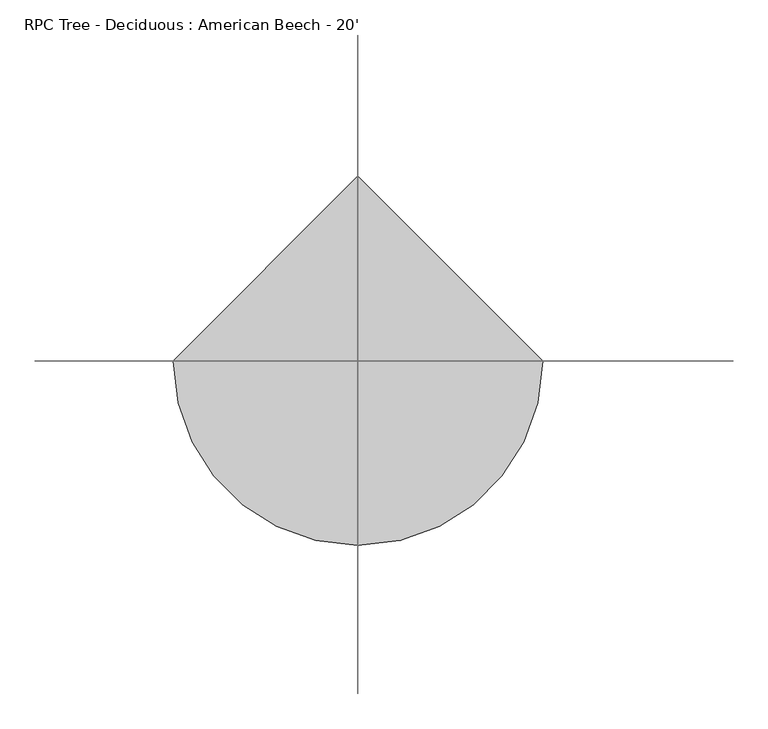
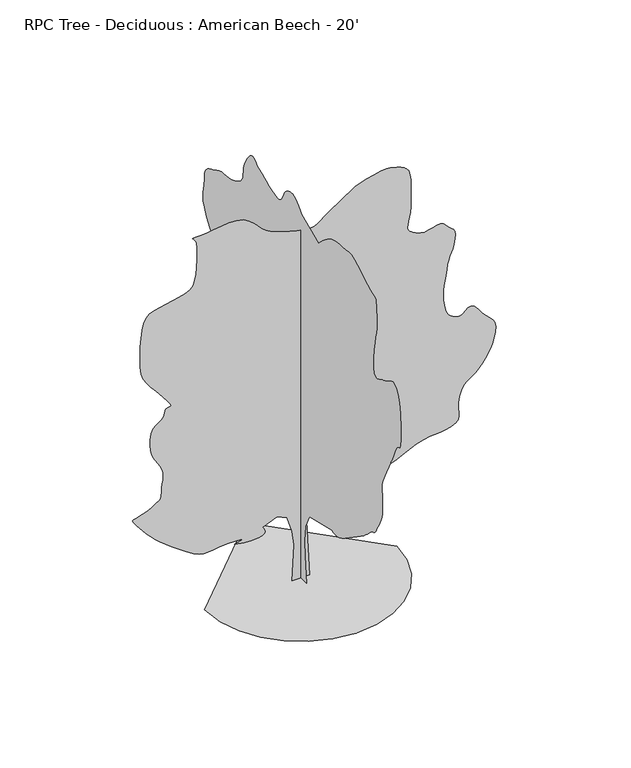
"""IFC4 building model written with IfcOpenShell, lengths in millimetres: geographic element geometry, RPC Tree - Deciduous : American Beech - 20'."""

from ifc_helpers import new_model, si_unit, origin, place, context, project, spatial, triangles, source, transform, mapped, element, save


def rpc_tree_deciduous_american_beech_20_b3c041c8(model_context):
    return source(origin(), model_context, "Body", "Tessellation", [
        triangles([(0.0009889, 136.856581, 0.0), (0.0009889, -149.8547884, 0.0), (0.0009889, -111.6264895, 420.510052), (0.0009889, -102.0697236, 659.4353302), (0.0009889, -121.1832463, 898.3606447), (0.0009889, -235.8678885, 1118.172373), (0.0009889, -818.8458761, 1261.5275036), (0.0009889, -849.9431059, 1249.7139805), (0.0009889, -883.2933231, 1240.7427258), (0.0009889, -921.1596891, 1237.4533916), (0.0009889, -965.7976622, 1242.6934788), (0.0009889, -1019.4603024, 1259.3000233), (0.0009889, -1084.4081549, 1290.1152935), (0.0009889, -1162.8992941, 1337.984174), (0.0009889, -1478.2811337, 1557.7959023), (0.0009889, -1522.8632961, 1589.1420994), (0.0009889, -1566.942437, 1618.9819931), (0.0009889, -1611.1893002, 1649.3249084), (0.0009889, -1656.2718681, 1682.1772636), (0.0009889, -1702.8579781, 1719.5406807), (0.0009889, -1751.6183739, 1763.4243393), (0.0009889, -1803.2210381, 1815.834803), (0.0009889, -1847.9404015, 1858.0191467), (0.0009889, -1878.9512993, 1877.1351311), (0.0009889, -1901.2702858, 1884.0440117), (0.0009889, -1919.9112991, 1889.616782), (0.0009889, -1939.8884228, 1904.7196392), (0.0009889, -1966.2180656, 1940.2161644), (0.0009889, -2003.916782, 2006.9774963), (0.0009889, -2044.9607883, 2083.2080177), (0.0009889, -2078.313549, 2145.2324295), (0.0009889, -2104.4754696, 2201.0692829), (0.0009889, -2123.9521877, 2258.7475937), (0.0009889, -2137.244109, 2326.2862038), (0.0009889, -2144.8488773, 2411.7141289), (0.0009889, -2147.2746014, 2523.0550072), (0.0009889, -2142.5373905, 2624.8889076), (0.0009889, -2132.7863869, 2688.2873634), (0.0009889, -2124.7040314, 2730.9338882), (0.0009889, -2124.9835201, 2770.583503), (0.0009889, -2140.3072941, 2824.9394875), (0.0009889, -2177.3659332, 2911.7568626), (0.0009889, -2242.84464, 3048.6883301), (0.0009889, -2308.7119858, 3181.9621719), (0.0009889, -2348.5011269, 3259.3812836), (0.0009889, -2371.2366577, 3301.215358), (0.0009889, -2385.9484051, 3327.6567673), (0.0009889, -2401.6632889, 3358.9496246), (0.0009889, -2427.4088104, 3415.3121727), (0.0009889, -2472.2118896, 3516.9885246), (0.0009889, -2522.8114174, 3609.6476944), (0.0009889, -2561.0332123, 3645.1568642), (0.0009889, -2588.5669968, 3652.9040657), (0.0009889, -2607.0580193, 3662.3273277), (0.0009889, -2618.2087921, 3702.8402618), (0.0009889, -2623.669796, 3803.856189), (0.0009889, -2625.117382, 3994.8390083), (0.0009889, -2615.3639076, 4210.713913), (0.0009889, -2589.2271309, 4371.4450905), (0.0009889, -2551.406765, 4483.8402649), (0.0009889, -2506.5400269, 4554.7824463), (0.0009889, -2459.3391289, 4591.1043571), (0.0009889, -2414.4802391, 4599.6895889), (0.0009889, -2376.641851, 4587.3705734), (0.0009889, -2343.8477772, 4566.9491455), (0.0009889, -2310.8862717, 4546.8576393), (0.0009889, -2277.5893215, 4527.4521378), (0.0009889, -2243.7921112, 4509.0116936), (0.0009889, -2209.3243023, 4491.9426773), (0.0009889, -2174.0232594, 4476.5250137), (0.0009889, -2137.7164639, 4463.1392029), (0.0009889, -2096.4236355, 4443.6572525), (0.0009889, -2049.6139927, 4418.4858238), (0.0009889, -2002.3013283, 4400.6805153), (0.0009889, -1959.504958, 4403.2713455), (0.0009889, -1926.2359131, 4439.313913), (0.0009889, -1907.5110386, 4521.8132378), (0.0009889, -1908.3467434, 4663.8246277), (0.0009889, -1923.6450829, 4819.4253044), (0.0009889, -1942.954224, 4940.7356323), (0.0009889, -1963.266647, 5037.9669067), (0.0009889, -1981.572361, 5121.3298416), (0.0009889, -1994.8642822, 5201.0354416), (0.0009889, -2000.1296585, 5287.2429703), (0.0009889, -1994.3614059, 5390.1634323), (0.0009889, -1986.3653824, 5488.9190323), (0.0009889, -1983.048143, 5559.911792), (0.0009889, -1978.5625156, 5609.3407516), (0.0009889, -1967.0562412, 5643.3764648), (0.0009889, -1942.6748806, 5668.2429703), (0.0009889, -1899.5709709, 5690.0869858), (0.0009889, -1831.8926891, 5715.1063889), (0.0009889, -1748.4408062, 5751.9616974), (0.0009889, -1662.820015, 5800.5261749), (0.0009889, -1576.3582867, 5853.7903656), (0.0009889, -1490.4020508, 5904.6919098), (0.0009889, -1406.2848015, 5946.2207703), (0.0009889, -1325.3426491, 5971.3924896), (0.0009889, -1248.913884, 5973.1447083), (0.0009889, -1174.2403896, 5963.3406555), (0.0009889, -1098.5636135, 5956.711409), (0.0009889, -1023.222064, 5950.5641098), (0.0009889, -949.5518515, 5942.2588028), (0.0009889, -878.8914843, 5929.1264648), (0.0009889, -812.5771454, 5908.4509827), (0.0009889, -751.9472706, 5877.5644958), (0.0009889, -697.9494038, 5841.2678741), (0.0009889, -649.9687569, 5805.9618896), (0.0009889, -607.0045916, 5771.4942261), (0.0009889, -568.0511189, 5737.7119858), (0.0009889, -532.1075644, 5704.4128555), (0.0009889, -498.1706097, 5671.4433563), (0.0009889, -465.2369368, 5638.6523346), (0.0009889, -16.056217, 5829.7871796), (0.0009889, 22.8405617, 5872.4339951), (0.0009889, 61.6537222, 5913.023378), (0.0009889, 100.2998553, 5949.3961578), (0.0009889, 138.6950317, 5979.5204819), (0.0009889, 176.7559443, 6001.2883392), (0.0009889, 214.3990318, 6012.5911377), (0.0009889, 251.5404602, 6011.3720261), (0.0009889, 287.2056524, 6002.4312927), (0.0009889, 320.3628219, 5991.305809), (0.0009889, 350.8454089, 5977.0055191), (0.0009889, 378.4856913, 5958.5397858), (0.0009889, 403.1160919, 5934.892392), (0.0009889, 424.5689612, 5905.047702), (0.0009889, 442.6817001, 5868.0144974), (0.0009889, 459.9562634, 5826.9425858), (0.0009889, 480.2407084, 5787.547316), (0.0009889, 505.3740581, 5752.6727005), (0.0009889, 537.1926464, 5725.138916), (0.0009889, 577.5380399, 5707.7911377), (0.0009889, 628.2491524, 5703.5239563), (0.0009889, 691.1650068, 5715.1063889), (0.0009889, 759.6790661, 5736.9754028), (0.0009889, 826.1890326, 5761.3593796), (0.0009889, 891.0251186, 5787.8263687), (0.0009889, 954.5251671, 5815.9694183), (0.0009889, 1017.0218611, 5845.3577408), (0.0009889, 1078.8506453, 5875.5832214), (0.0009889, 1140.3440575, 5906.2412338), (0.0009889, 1169.0715191, 5932.3524307), (0.0009889, 1198.1316639, 5955.3649796), (0.0009889, 1227.8624073, 5972.2052307), (0.0009889, 1258.5938164, 5979.7489563), (0.0009889, 1290.6664227, 5974.9230881), (0.0009889, 1324.4078224, 5954.6539764), (0.0009889, 1360.1557858, 5915.7918137), (0.0009889, 1395.1799561, 5868.217392), (0.0009889, 1426.1908539, 5822.9544571), (0.0009889, 1452.6880737, 5778.8856354), (0.0009889, 1474.1715008, 5734.7912338), (0.0009889, 1490.1379681, 5689.5538788), (0.0009889, 1500.0845993, 5641.9538773), (0.0009889, 1503.510989, 5590.8494385), (0.0009889, 1507.2168674, 5539.3380478), (0.0009889, 1519.1142517, 5491.1793594), (0.0009889, 1540.3740005, 5446.1704788), (0.0009889, 1572.1672634, 5404.1846695), (0.0009889, 1615.6596668, 5365.0428726), (0.0009889, 1672.0274471, 5328.5689362), (0.0009889, 1742.4363762, 5294.5832199), (0.0009889, 1817.5288857, 5269.1836075), (0.0009889, 1887.9378147, 5255.1373718), (0.0009889, 1954.8363476, 5247.4407486), (0.0009889, 2019.3956337, 5241.0911362), (0.0009889, 2082.7839157, 5231.0580276), (0.0009889, 2146.1721977, 5212.3382401), (0.0009889, 2210.7313385, 5179.9024292), (0.0009889, 2276.3498623, 5145.3580261), (0.0009889, 2340.1267834, 5118.8404587), (0.0009889, 2399.0573433, 5093.1356323), (0.0009889, 2450.1315514, 5061.106192), (0.0009889, 2490.3372368, 5015.5136261), (0.0009889, 2516.667025, 4949.193837), (0.0009889, 2526.1132507, 4854.9597633), (0.0009889, 2532.46577, 4758.008123), (0.0009889, 2546.5044479, 4681.9348595), (0.0009889, 2560.7285797, 4617.2411339), (0.0009889, 2567.5865913, 4554.3760757), (0.0009889, 2559.5600464, 4483.8402649), (0.0009889, 2529.1232414, 4396.0578323), (0.0009889, 2468.7702393, 4281.5543564), (0.0009889, 2394.0992157, 4166.6192207), (0.0009889, 2326.6139454, 4078.2525215), (0.0009889, 2267.6553349, 4007.9707649), (0.0009889, 2218.5596397, 3947.1884285), (0.0009889, 2180.6679119, 3887.4223091), (0.0009889, 2155.3111748, 3820.1377533), (0.0009889, 2143.8328056, 3736.8001076), (0.0009889, 2149.4334812, 3646.0204742), (0.0009889, 2171.0820145, 3561.7686401), (0.0009889, 2203.7667927, 3483.5112076), (0.0009889, 2242.4687908, 3410.790937), (0.0009889, 2282.1714546, 3343.1000107), (0.0009889, 2317.8662235, 3279.9047401), (0.0009889, 2344.5311657, 3220.7225967), (0.0009889, 2370.3577869, 3180.6921913), (0.0009889, 2402.5396889, 3164.8934464), (0.0009889, 2434.5538685, 3157.7813805), (0.0009889, 2459.8827003, 3143.8113029), (0.0009889, 2472.0037628, 3107.4638123), (0.0009889, 2464.3963783, 3033.1433487), (0.0009889, 2430.5432121, 2905.3305107), (0.0009889, 2383.9011463, 2761.3378464), (0.0009889, 2340.6017544, 2643.9136185), (0.0009889, 2298.1379219, 2545.7425758), (0.0009889, 2254.0028252, 2459.415287), (0.0009889, 2205.6894951, 2377.6095245), (0.0009889, 2150.6857304, 2292.9614937), (0.0009889, 2086.4897942, 2198.1177189), (0.0009889, 2022.098085, 2102.5196297), (0.0009889, 1968.0723129, 2019.6267242), (0.0009889, 1924.2446102, 1948.102747), (0.0009889, 1890.4447838, 1886.6067913), (0.0009889, 1866.5103436, 1833.8078339), (0.0009889, 1852.2735672, 1788.3620613), (0.0009889, 1847.564407, 1748.9361248), (0.0009889, 1851.5776794, 1721.8800728), (0.0009889, 1860.940044, 1709.2029396), (0.0009889, 1871.6386642, 1703.0459026), (0.0009889, 1879.6624477, 1695.5504299), (0.0009889, 1881.0010288, 1678.8600243), (0.0009889, 1871.6386642, 1645.1186245), (0.0009889, 1847.564407, 1586.4675533), (0.0009889, 1827.5314728, 1524.5828133), (0.0009889, 1825.3850922, 1482.2587978), (0.0009889, 1829.7590984, 1453.3104195), (0.0009889, 1829.2865982, 1431.547649), (0.0009889, 1812.5961926, 1410.7907764), (0.0009889, 1768.3214241, 1384.8497726), (0.0009889, 1685.0958355, 1347.5421661), (0.0009889, 1594.399918, 1309.4244347), (0.0009889, 1528.281134, 1282.5080544), (0.0009889, 1476.2059696, 1262.7823689), (0.0009889, 1427.6412014, 1246.2316349), (0.0009889, 1372.05317, 1228.8453415), (0.0009889, 1298.9138844, 1206.6102161), (0.0009889, 1197.6871416, 1175.5154572), (0.0009889, 1096.069289, 1145.7009253), (0.0009889, 1022.5387482, 1127.7557997), (0.0009889, 967.7331545, 1118.3400227), (0.0009889, 922.2874546, 1114.10329), (0.0009889, 876.8442255, 1111.7080873), (0.0009889, 822.0360884, 1107.806654), (0.0009889, 748.5055475, 1099.0588594), (0.0009889, 662.4935011, 1085.0990284), (0.0009889, 576.4788749, 1068.1292793), (0.0009889, 490.4667558, 1048.6551046), (0.0009889, 404.4521296, 1027.1717503), (0.0009889, 318.4400468, 1004.1847086), (0.0009889, 232.4266923, 980.1943851), (0.0009889, 146.4133378, 955.7037289), (136.1842383, 0.0003154, 0.014068), (-131.4120823, 0.0003154, 0.014068), (-102.7410489, 0.0002819, 563.8778998), (-131.4120823, 0.0002692, 793.2477293), (-207.8684348, 0.0002549, 1032.1729712), (-360.7819027, 0.0002501, 1108.6296415), (-580.5936673, 0.0002549, 1013.0594576), (-562.704425, 0.0002564, 988.5662579), (-548.0765751, 0.000258, 964.5784779), (-539.9688578, 0.0002596, 941.5914362), (-541.6401947, 0.0002612, 920.1080818), (-556.3518694, 0.0002628, 900.6313637), (-587.3627672, 0.0002628, 883.6641581), (-637.9342443, 0.0002644, 869.704327), (-697.421093, 0.0002644, 860.4815615), (-753.4001616, 0.0002644, 856.775683), (-806.4506298, 0.0002644, 857.667271), (-857.1617786, 0.0002644, 862.2366869), (-906.117802, 0.0002644, 869.5645826), (-953.9028214, 0.0002628, 878.731465), (-1001.1011759, 0.0002628, 888.8178406), (-953.2881786, 0.0002628, 900.9945683), (-913.501581, 0.0002612, 912.5008427), (-889.7601522, 0.0002612, 922.6710068), (-890.0954515, 0.0002596, 930.8345346), (-922.5287189, 0.0002596, 936.3235165), (-995.0838833, 0.0002596, 938.4698244), (-1115.7848007, 0.0002596, 936.6028599), (-1242.9524746, 0.0002612, 927.8271601), (-1337.3542706, 0.0002612, 914.3677345), (-1410.6891838, 0.0002612, 903.2500992), (-1474.6617325, 0.0002612, 901.4949738), (-1540.9759987, 0.0002612, 916.12286), (-1621.3340298, 0.0002596, 954.1568756), (-1727.4351116, 0.0002549, 1022.614979), (-1845.0726986, 0.0002501, 1105.8432564), (-1952.34711, 0.0002453, 1184.0549795), (-2049.4209812, 0.0002405, 1258.0858532), (-2136.46436, 0.0002373, 1328.7765965), (-2213.6472942, 0.0002326, 1396.9554291), (-2281.1300938, 0.0002278, 1463.4653229), (-2339.0852772, 0.0002246, 1529.1396572), (-2391.8031349, 0.0002214, 1592.6651402), (-2441.3431343, 0.0002166, 1651.1791557), (-2484.5309052, 0.0002134, 1703.170459), (-2518.1884438, 0.0002118, 1747.1378334), (-2539.1409439, 0.0002103, 1781.577737), (-2544.218541, 0.0002087, 1804.9838665), (-2530.2254997, 0.0002071, 1815.8500637), (-2498.742247, 0.0002071, 1822.7308937), (-2456.2227493, 0.0002071, 1834.628278), (-2406.8475655, 0.0002055, 1850.7065117), (-2354.8003063, 0.0002039, 1870.1272739), (-2304.2568798, 0.0002023, 1892.0551506), (-2259.3978447, 0.0002023, 1915.6542915), (-2224.401725, 0.0002007, 1940.091608), (-2196.9849392, 0.0001991, 1958.6464348), (-2172.4078056, 0.0001991, 1969.1798035), (-2151.1759621, 0.0001975, 1977.7066086), (-2133.7896687, 0.0001975, 1990.2439247), (-2120.7518017, 0.0001959, 2012.8144947), (-2112.5602959, 0.0001927, 2051.4326317), (-2109.7180275, 0.0001895, 2112.118317), (-2105.7607109, 0.0001864, 2181.0514641), (-2096.7894562, 0.0001816, 2242.2935108), (-2087.1476028, 0.0001784, 2298.6891964), (-2081.1861935, 0.0001752, 2353.0781731), (-2083.2487129, 0.000172, 2408.3028545), (-2097.6809715, 0.0001688, 2467.2028931), (-2128.8315411, 0.0001641, 2532.6259346), (-2168.3971493, 0.0001609, 2596.7202782), (-2204.2849297, 0.0001577, 2653.2860115), (-2235.1560104, 0.0001545, 2707.6675758), (-2259.6771881, 0.0001513, 2765.2239464), (-2276.5047947, 0.0001465, 2831.3149704), (-2284.3076614, 0.0001418, 2911.2740433), (-2281.7447365, 0.000137, 3010.4865921), (-2264.5514545, 0.0001306, 3102.7902603), (-2233.1494469, 0.0001274, 3164.9948936), (-2193.2231049, 0.0001242, 3206.8286774), (-2150.4520237, 0.0001226, 3237.9439293), (-2110.525827, 0.0001211, 3268.0682533), (-2079.123674, 0.0001179, 3306.8795471), (-2061.9330082, 0.0001147, 3364.0804161), (-2043.9599773, 0.0001131, 3413.0262657), (-2014.1200836, 0.0001115, 3431.3396828), (-1983.9422745, 0.0001115, 3435.3019409), (-1964.9684326, 0.0001099, 3441.0931572), (-1968.7301216, 0.0001099, 3464.9437363), (-2006.7641373, 0.0001051, 3523.0843735), (-2090.6020432, 9.88e-05, 3631.6948952), (-2191.4121689, 9.24e-05, 3753.7165169), (-2273.3296978, 8.6e-05, 3849.6778107), (-2337.3582024, 8.12e-05, 3932.1009773), (-2384.5031445, 7.65e-05, 4013.5079269), (-2415.7654804, 7.17e-05, 4106.47202), (-2432.1484921, 6.37e-05, 4223.4898773), (-2434.6554611, 5.42e-05, 4377.1345688), (-2429.5297565, 4.46e-05, 4541.5998207), (-2420.5585018, 3.66e-05, 4683.0016548), (-2405.0643894, 3.03e-05, 4801.6705742), (-2380.3781055, 2.39e-05, 4897.9365005), (-2343.822488, 1.91e-05, 4972.1558075), (-2292.720084, 1.59e-05, 5024.6066757), (-2224.401725, 1.43e-05, 5055.6710587), (-2138.4149677, 1.27e-05, 5074.7972168), (-2040.8941761, 1.27e-05, 5092.7292618), (-1939.0274288, 1.11e-05, 5111.8554199), (-1840.0028046, 9.6e-06, 5134.487178), (-1751.0088181, 8e-06, 5162.9604401), (-1679.2334026, 6.4e-06, 5199.612854), (-1631.8649277, 3.2e-06, 5246.8314835), (-1604.1128426, -1.6e-06, 5316.4272354), (-1585.3905842, -6.4e-06, 5411.6010773), (-1574.1890877, -1.27e-05, 5521.6594757), (-1569.0075726, -2.07e-05, 5635.9088974), (-1568.336974, -2.71e-05, 5743.6302292), (-1570.6788368, -3.19e-05, 5834.1305191), (-1574.524387, -3.5e-05, 5896.690654), (-1585.918895, -3.82e-05, 5936.1626633), (-1606.0102558, -3.98e-05, 5965.4230865), (-1625.9315689, -4.14e-05, 5985.9718323), (-1636.825526, -4.14e-05, 5999.3576431), (-1629.8329296, -4.3e-05, 6007.0286865), (-1596.0890591, -4.3e-05, 6010.559285), (-1526.7393677, -4.3e-05, 6011.3976059), (-1428.7715103, -4.3e-05, 6017.8233765), (-1318.7690678, -4.46e-05, 6032.4538788), (-1202.2439129, -4.46e-05, 6048.2529144), (-1084.7180197, -4.46e-05, 6058.184285), (-971.7057318, -4.46e-05, 6055.263533), (-868.7238636, -4.46e-05, 6032.4538788), (-781.2893749, -4.14e-05, 5982.7208679), (-714.8937183, -3.66e-05, 5922.6245361), (-665.5465851, -3.34e-05, 5871.6974121), (-624.5610781, -3.19e-05, 5827.4756927), (-583.2403444, -2.87e-05, 5787.445578), (-532.8924365, -2.71e-05, 5749.0915237), (-464.8228995, -2.39e-05, 5709.8735687), (-370.3373878, -2.23e-05, 5667.3284912), (-260.8632923, -1.91e-05, 5627.3745346), (-155.7366604, -1.75e-05, 5596.9449966), (-58.1322665, -1.59e-05, 5575.0504028), (28.7726351, -1.59e-05, 5560.6739548), (101.8020074, -1.59e-05, 5552.8255966), (157.7788323, -1.43e-05, 5550.4629501), (193.5270681, -1.59e-05, 5552.6477005), (219.2725352, -1.59e-05, 5560.6233765), (247.3583572, -1.59e-05, 5575.4311935), (277.7847885, -1.75e-05, 5595.7770447), (310.5508118, -1.91e-05, 5620.2877579), (345.6587342, -2.07e-05, 5647.6692261), (383.1059761, -2.23e-05, 5676.5232788), (422.8950809, -2.39e-05, 5705.555809), (805.1781057, -3.98e-05, 5963.5947098), (830.3647951, -3.98e-05, 5972.992392), (896.679134, -4.14e-05, 5996.5892075), (990.2426817, -4.3e-05, 6027.5518524), (1097.1817938, -4.62e-05, 6058.9970261), (1203.6180296, -4.62e-05, 6084.1175858), (1295.67789, -4.78e-05, 6096.0046509), (1359.4853325, -4.78e-05, 6087.8516602), (1407.4912685, -4.62e-05, 6070.6556168), (1459.1777939, -4.46e-05, 6056.8128571), (1511.1996185, -4.46e-05, 6041.4457718), (1560.2089817, -4.3e-05, 6019.7540726), (1602.8682964, -4.14e-05, 5986.835733), (1635.8299473, -3.82e-05, 5937.8898834), (1655.7537312, -3.34e-05, 5868.0394958), (1665.3091072, -2.87e-05, 5789.7820633), (1670.1859898, -2.55e-05, 5717.2399796), (1671.5500053, -2.07e-05, 5647.8471222), (1670.5746288, -1.75e-05, 5579.1396881), (1668.4282482, -1.27e-05, 5508.6038773), (1666.2844837, -8e-06, 5433.699147), (1665.3091072, -3.2e-06, 5351.9622757), (1660.2367424, 1.6e-06, 5270.5806152), (1648.1463467, 6.4e-06, 5198.4187408), (1633.7114719, 9.6e-06, 5135.2743393), (1621.6186054, 1.27e-05, 5081.0200928), (1616.5487114, 1.59e-05, 5035.4269455), (1623.1807194, 1.75e-05, 4998.368161), (1646.1955936, 1.91e-05, 4969.6664246), (1678.4054008, 2.07e-05, 4946.8317719), (1709.6119263, 2.23e-05, 4927.324823), (1739.9826015, 2.23e-05, 4910.992099), (1769.6829689, 2.39e-05, 4897.6824463), (1798.8852562, 2.39e-05, 4887.1923889), (1827.7499187, 2.55e-05, 4879.3946091), (1856.4493298, 2.55e-05, 4874.0862122), (1893.0609032, 2.55e-05, 4877.1087021), (1942.2125542, 2.39e-05, 4889.9864044), (1998.8851124, 2.39e-05, 4906.1918106), (2058.0671104, 2.23e-05, 4919.2474091), (2114.7396687, 2.23e-05, 4922.5745316), (2163.8911743, 2.39e-05, 4909.6968292), (2200.5028931, 2.55e-05, 4874.0862122), (2230.4850746, 2.71e-05, 4834.208123), (2261.3003448, 2.87e-05, 4807.6649757), (2290.2766285, 3.03e-05, 4786.8368866), (2314.7419956, 3.19e-05, 4763.9769447), (2332.0165226, 3.34e-05, 4731.4396866), (2339.4282795, 3.66e-05, 4681.5031998), (2334.3025749, 4.14e-05, 4606.4970222), (2319.8956055, 4.62e-05, 4526.9440292), (2302.1485783, 4.94e-05, 4463.951944), (2282.3925167, 5.26e-05, 4410.6627548), (2261.9683273, 5.57e-05, 4360.1928703), (2242.2147366, 5.89e-05, 4305.7098587), (2224.4652386, 6.37e-05, 4240.3809975), (2210.0608852, 6.85e-05, 4157.3229858), (2196.9087811, 7.33e-05, 4068.4481781), (2183.2562714, 7.8e-05, 3988.0827347), (2170.9397266, 8.28e-05, 3913.0762665), (2161.8007496, 8.76e-05, 3840.2289688), (2157.6783268, 9.08e-05, 3766.3913246), (2160.4088287, 9.56e-05, 3688.3876556), (2171.831242, 0.0001003, 3603.0181572), (2189.9719952, 0.0001051, 3525.0147789), (2211.6203831, 0.0001083, 3468.2711494), (2236.7791672, 0.0001115, 3428.240744), (2265.4506729, 0.0001131, 3400.402327), (2297.6324295, 0.0001147, 3380.2602425), (2333.3271984, 0.0001147, 3363.2673843), (2372.5296021, 0.0001163, 3344.9795471), (2412.5675652, 0.0001163, 3342.4901642), (2451.7724396, 0.0001147, 3366.0869797), (2491.642971, 0.0001131, 3400.8848557), (2533.6901138, 0.0001115, 3432.0253967), (2579.4227875, 0.0001099, 3444.5728867), (2630.3246223, 0.0001115, 3423.7195084), (2687.906282, 0.0001163, 3354.5298363), (2749.8568611, 0.0001211, 3269.9730789), (2810.1313797, 0.0001242, 3206.9557045), (2864.6905495, 0.0001274, 3156.6637161), (2909.5976921, 0.0001306, 3110.2325386), (2940.7635223, 0.0001338, 3058.7720169), (2954.2254913, 0.000137, 2993.4178665), (2945.9451828, 0.0001434, 2905.3557999), (2924.1520363, 0.0001481, 2810.6139084), (2899.209082, 0.0001529, 2729.079641), (2870.2277115, 0.0001577, 2657.6040619), (2836.3948929, 0.0001609, 2592.9612053), (2796.8723053, 0.0001641, 2531.9858574), (2750.8474983, 0.0001688, 2471.5235596), (2697.4568619, 0.000172, 2408.3842449), (2642.4404526, 0.0001752, 2354.2186558), (2591.9196991, 0.0001784, 2316.7713776), (2545.7425758, 0.00018, 2287.0127289), (2503.7637428, 0.0001816, 2255.9181152), (2465.7858284, 0.0001832, 2214.4575645), (2431.6531734, 0.000188, 2153.606773), (2401.2011078, 0.0001927, 2064.3332977), (2384.7901909, 0.0001991, 1965.7532684), (2385.7654221, 0.0002039, 1881.8849865), (2393.4261463, 0.0002071, 1811.0570423), (2397.0760689, 0.0002118, 1751.5981716), (2386.0143894, 0.000215, 1701.8343487), (2349.5424877, 0.0002166, 1660.0945999), (2276.9594181, 0.0002182, 1624.7096958), (2189.7484623, 0.0002198, 1601.1638947), (2111.7322941, 0.0002214, 1590.8261536), (2035.7202187, 0.0002214, 1585.8401207), (1954.5264828, 0.0002214, 1578.3445026), (1860.9630077, 0.000223, 1560.4858543), (1747.8389534, 0.0002246, 1524.4025917), (1607.9660957, 0.0002294, 1462.2385082), (1455.667543, 0.0002326, 1390.7425816), (1311.7282185, 0.0002357, 1331.4512878), (1178.6524023, 0.0002389, 1283.6941738), (1058.9547667, 0.0002421, 1246.8031116), (955.1372663, 0.0002437, 1220.1102642), (869.7094139, 0.0002437, 1202.9449602), (805.1781057, 0.0002453, 1194.641688), (403.7815673, 0.0002453, 1185.0862392), (107.513205, 0.0002485, 1137.3011473), (88.3996914, 0.0002628, 879.2597757), (-1453.7574852, 0.0, 0.0120292), (-1415.3246567, -333.1060121, 0.0120292), (-1305.8708725, -639.0085974, 0.0120292), (-1134.1566444, -908.9473532, 0.0120292), (-908.9473532, -1134.1566444, 0.0120292), (-639.0085974, -1305.8708725, 0.0120292), (-333.1060121, -1415.3246567, 0.0120292), (6.35e-05, -1453.7574852, 0.0120292), (333.1060121, -1415.3246567, 0.0120292), (639.0085974, -1305.8708725, 0.0120292), (908.9473532, -1134.1566444, 0.0120292), (1134.1566444, -908.9473532, 0.0120292), (1305.8708725, -639.0085974, 0.0120292), (1415.3246567, -333.1060121, 0.0120292), (1453.7574852, 0.0001274, 0.0120292), (-0.0001906, 1453.7574852, 0.0120292)], [[1, 2, 3], [254, 1, 3], [254, 3, 4], [254, 4, 5], [254, 5, 6], [53, 54, 55], [52, 53, 55], [201, 202, 203], [201, 203, 204], [200, 201, 204], [222, 223, 224], [52, 55, 56], [200, 204, 205], [199, 200, 205], [253, 254, 6], [221, 222, 224], [221, 224, 225], [229, 230, 231], [229, 231, 232], [228, 229, 232], [228, 232, 233], [227, 228, 233], [252, 253, 6], [221, 225, 226], [220, 221, 226], [199, 205, 206], [198, 199, 206], [62, 63, 64], [61, 62, 64], [61, 64, 65], [60, 61, 65], [60, 65, 66], [59, 60, 66], [59, 66, 67], [59, 67, 68], [58, 59, 68], [58, 68, 69], [58, 69, 70], [57, 58, 70], [57, 70, 71], [57, 71, 72], [57, 72, 73], [57, 73, 74], [56, 57, 74], [52, 56, 74], [51, 52, 74], [50, 51, 74], [50, 74, 75], [49, 50, 75], [48, 49, 75], [47, 48, 75], [46, 47, 75], [45, 46, 75], [44, 45, 75], [43, 44, 75], [42, 43, 75], [42, 75, 76], [41, 42, 76], [227, 233, 234], [226, 227, 234], [220, 226, 234], [219, 220, 234], [219, 234, 235], [219, 235, 236], [219, 236, 237], [218, 219, 237], [218, 237, 238], [218, 238, 239], [218, 239, 240], [217, 218, 240], [217, 240, 241], [217, 241, 242], [217, 242, 243], [217, 243, 244], [217, 244, 245], [217, 245, 246], [216, 217, 246], [216, 246, 247], [215, 216, 247], [215, 247, 248], [251, 252, 6], [88, 89, 90], [88, 90, 91], [87, 88, 91], [87, 91, 92], [86, 87, 92], [86, 92, 93], [85, 86, 93], [84, 85, 93], [84, 93, 94], [83, 84, 94], [82, 83, 94], [81, 82, 94], [81, 94, 95], [80, 81, 95], [80, 95, 96], [80, 96, 97], [80, 97, 98], [80, 98, 99], [80, 99, 100], [80, 100, 101], [80, 101, 102], [80, 102, 103], [80, 103, 104], [80, 104, 105], [80, 105, 106], [80, 106, 107], [80, 107, 108], [80, 108, 109], [80, 109, 110], [80, 110, 111], [80, 111, 112], [79, 80, 112], [79, 112, 113], [78, 79, 113], [77, 78, 113], [76, 77, 113], [41, 76, 113], [40, 41, 113], [40, 113, 114], [39, 40, 114], [198, 206, 207], [197, 198, 207], [196, 197, 207], [196, 207, 208], [195, 196, 208], [195, 208, 209], [195, 209, 210], [195, 210, 211], [194, 195, 211], [194, 211, 212], [194, 212, 213], [193, 194, 213], [193, 213, 214], [214, 215, 248], [193, 214, 248], [193, 248, 249], [192, 193, 249], [192, 249, 250], [192, 250, 251], [192, 251, 6], [192, 6, 7], [191, 192, 7], [190, 191, 7], [189, 190, 7], [38, 39, 114], [37, 38, 114], [36, 37, 114], [35, 36, 114], [34, 35, 114], [33, 34, 114], [32, 33, 114], [31, 32, 114], [30, 31, 114], [29, 30, 114], [28, 29, 114], [27, 28, 114], [26, 27, 114], [25, 26, 114], [24, 25, 114], [23, 24, 114], [22, 23, 114], [21, 22, 114], [20, 21, 114], [19, 20, 114], [18, 19, 114], [17, 18, 114], [16, 17, 114], [15, 16, 114], [14, 15, 114], [13, 14, 114], [12, 13, 114], [11, 12, 114], [10, 11, 114], [9, 10, 114], [8, 9, 114], [7, 8, 114], [189, 7, 114], [188, 189, 114], [188, 114, 115], [188, 115, 116], [188, 116, 117], [188, 117, 118], [188, 118, 119], [188, 119, 120], [188, 120, 121], [146, 147, 148], [145, 146, 148], [144, 145, 148], [144, 148, 149], [143, 144, 149], [143, 149, 150], [142, 143, 150], [142, 150, 151], [142, 151, 152], [141, 142, 152], [141, 152, 153], [141, 153, 154], [141, 154, 155], [141, 155, 156], [140, 141, 156], [140, 156, 157], [139, 140, 157], [138, 139, 157], [138, 157, 158], [137, 138, 158], [137, 158, 159], [136, 137, 159], [135, 136, 159], [135, 159, 160], [134, 135, 160], [134, 160, 161], [174, 175, 176], [173, 174, 176], [173, 176, 177], [172, 173, 177], [171, 172, 177], [171, 177, 178], [170, 171, 178], [170, 178, 179], [169, 170, 179], [168, 169, 179], [167, 168, 179], [166, 167, 179], [165, 166, 179], [165, 179, 180], [165, 180, 181], [165, 181, 182], [165, 182, 183], [165, 183, 184], [165, 184, 185], [165, 185, 186], [165, 186, 187], [164, 165, 187], [164, 187, 188], [163, 164, 188], [162, 163, 188], [161, 162, 188], [134, 161, 188], [133, 134, 188], [132, 133, 188], [125, 126, 127], [124, 125, 127], [124, 127, 128], [123, 124, 128], [122, 123, 128], [121, 122, 128], [121, 128, 129], [121, 129, 130], [121, 130, 131], [188, 121, 131], [132, 188, 131], [274, 275, 276], [531, 255, 256], [531, 256, 257], [531, 257, 258], [531, 258, 259], [530, 531, 259], [376, 377, 378], [376, 378, 379], [375, 376, 379], [273, 274, 276], [273, 276, 277], [375, 379, 380], [374, 375, 380], [273, 277, 278], [272, 273, 278], [301, 302, 303], [301, 303, 304], [300, 301, 304], [300, 304, 305], [299, 300, 305], [299, 305, 306], [298, 299, 306], [298, 306, 307], [297, 298, 307], [297, 307, 308], [271, 272, 278], [296, 297, 308], [296, 308, 309], [373, 374, 380], [373, 380, 381], [372, 373, 381], [295, 296, 309], [295, 309, 310], [294, 295, 310], [294, 310, 311], [294, 311, 312], [294, 312, 313], [293, 294, 313], [293, 313, 314], [292, 293, 314], [271, 278, 279], [291, 292, 314], [530, 259, 260], [372, 381, 382], [371, 372, 382], [291, 314, 315], [290, 291, 315], [371, 382, 383], [370, 371, 383], [370, 383, 384], [369, 370, 384], [369, 384, 385], [369, 385, 386], [369, 386, 387], [369, 387, 388], [369, 388, 389], [369, 389, 390], [368, 369, 390], [368, 390, 391], [367, 368, 391], [367, 391, 392], [367, 392, 393], [366, 367, 393], [366, 393, 394], [270, 271, 279], [366, 394, 395], [338, 339, 340], [338, 340, 341], [289, 290, 315], [483, 484, 485], [483, 485, 486], [482, 483, 486], [481, 482, 486], [481, 486, 487], [480, 481, 487], [288, 289, 315], [287, 288, 315], [286, 287, 315], [285, 286, 315], [284, 285, 315], [283, 284, 315], [282, 283, 315], [282, 315, 316], [281, 282, 316], [281, 316, 317], [281, 317, 318], [281, 318, 319], [281, 319, 320], [280, 281, 320], [280, 320, 321], [279, 280, 321], [279, 321, 322], [480, 487, 488], [264, 265, 266], [263, 264, 266], [263, 266, 267], [262, 263, 267], [262, 267, 268], [261, 262, 268], [261, 268, 269], [261, 269, 270], [261, 270, 279], [261, 279, 322], [260, 261, 322], [530, 260, 322], [530, 322, 323], [529, 530, 323], [529, 323, 324], [366, 395, 396], [365, 366, 396], [337, 338, 341], [337, 341, 342], [529, 324, 325], [528, 529, 325], [527, 528, 325], [526, 527, 325], [525, 526, 325], [524, 525, 325], [523, 524, 325], [522, 523, 325], [521, 522, 325], [521, 325, 326], [521, 326, 327], [521, 327, 328], [521, 328, 329], [521, 329, 330], [521, 330, 331], [521, 331, 332], [521, 332, 333], [521, 333, 334], [521, 334, 335], [521, 335, 336], [521, 336, 337], [521, 337, 342], [520, 521, 342], [520, 342, 343], [519, 520, 343], [518, 519, 343], [518, 343, 344], [517, 518, 344], [449, 450, 451], [448, 449, 451], [448, 451, 452], [447, 448, 452], [446, 447, 452], [446, 452, 453], [516, 517, 344], [515, 516, 344], [514, 515, 344], [513, 514, 344], [512, 513, 344], [511, 512, 344], [510, 511, 344], [509, 510, 344], [508, 509, 344], [507, 508, 344], [506, 507, 344], [505, 506, 344], [504, 505, 344], [503, 504, 344], [502, 503, 344], [501, 502, 344], [500, 501, 344], [499, 500, 344], [498, 499, 344], [497, 498, 344], [496, 497, 344], [495, 496, 344], [494, 495, 344], [493, 494, 344], [492, 493, 344], [491, 492, 344], [490, 491, 344], [489, 490, 344], [488, 489, 344], [480, 488, 344], [479, 480, 344], [478, 479, 344], [477, 478, 344], [476, 477, 344], [475, 476, 344], [474, 475, 344], [473, 474, 344], [472, 473, 344], [471, 472, 344], [470, 471, 344], [469, 470, 344], [468, 469, 344], [467, 468, 344], [466, 467, 344], [465, 466, 344], [464, 465, 344], [463, 464, 344], [463, 344, 345], [462, 463, 345], [462, 345, 346], [461, 462, 346], [460, 461, 346], [459, 460, 346], [458, 459, 346], [457, 458, 346], [456, 457, 346], [455, 456, 346], [454, 455, 346], [453, 454, 346], [446, 453, 346], [445, 446, 346], [444, 445, 346], [443, 444, 346], [442, 443, 346], [441, 442, 346], [440, 441, 346], [439, 440, 346], [438, 439, 346], [437, 438, 346], [436, 437, 346], [435, 436, 346], [435, 346, 347], [435, 347, 348], [435, 348, 349], [435, 349, 350], [435, 350, 351], [435, 351, 352], [435, 352, 353], [435, 353, 354], [435, 354, 355], [435, 355, 356], [435, 356, 357], [435, 357, 358], [435, 358, 359], [435, 359, 360], [435, 360, 361], [435, 361, 362], [435, 362, 363], [435, 363, 364], [435, 364, 365], [435, 365, 396], [435, 396, 397], [435, 397, 398], [435, 398, 399], [435, 399, 400], [435, 400, 401], [435, 401, 402], [435, 402, 403], [435, 403, 404], [435, 404, 405], [435, 405, 406], [435, 406, 407], [435, 407, 408], [435, 408, 409], [434, 435, 409], [433, 434, 409], [432, 433, 409], [431, 432, 409], [430, 431, 409], [429, 430, 409], [429, 409, 410], [429, 410, 411], [429, 411, 412], [428, 429, 412], [428, 412, 413], [427, 428, 413], [426, 427, 413], [426, 413, 414], [425, 426, 414], [425, 414, 415], [425, 415, 416], [425, 416, 417], [424, 425, 417], [424, 417, 418], [423, 424, 418], [423, 418, 419], [422, 423, 419], [422, 419, 420], [421, 422, 420], [546, 547, 532], [545, 546, 532], [545, 532, 533], [544, 545, 533], [544, 533, 534], [544, 534, 535], [543, 544, 535], [542, 543, 535], [542, 535, 536], [542, 536, 537], [542, 537, 538], [542, 538, 539], [542, 539, 540], [542, 540, 541]], closed=False),
    ])


if __name__ == "__main__":
    model = new_model("IFC4")
    model_context = context("Model", 3, world=origin())
    ifc_project = project(units=[si_unit("LENGTHUNIT", "METRE", prefix="MILLI")], contexts=[model_context])
    site = spatial("IfcSite", under=ifc_project)
    building = spatial("IfcBuilding", under=site)
    placement = place(None, origin())
    rpc_tree_deciduous_american_beech_20_shape = rpc_tree_deciduous_american_beech_20_b3c041c8(model_context)
    element("IfcGeographicElement", 1, ObjectType="RPC Tree - Deciduous : American Beech - 20'", at=placement, inside=building, context=model_context, shape_type="MappedRepresentation", body=[
        mapped(rpc_tree_deciduous_american_beech_20_shape, transform((0.0, 0.0, 0.0), x_axis=(1.0, 0.0, 0.0), y_axis=(0.0, 1.0, 0.0), z_axis=(0.0, 0.0, 1.0))),
    ])
    save(model, "model.ifc")

# Revit data of these elements
# Type "RPC Tree - Deciduous : American Beech - 20'"
#   built-in parameter 1005198 = "{2, 15},{39, RPC-16-G1GQ-43Q0-7NP3-0000-ST1L-LVER-AU},{1, 0},{1, 0},{2, 13},{1, 8},{5, Color},{1, 0},{1, 0},{3, 0.8},{3, 0.8},{3, 0.8},{1, 8},{7, BBoxMin},{1, 0},{1, 0},{1, 0},{1, 0},{1, 0},{1, 8},{7, BBoxMax},{1, 0},{1, 0},{1, 0},{1, 0},{1, 0},{2, 11},{9, RPCTypeId},{1, 0},{1, 0},{39, RPC-16-G1GQ-43Q0-7NP3-0000-ST1L-LVER-AU},{1, 6},{14, RPCPlantHeight},{1, 0},{1, 0},{2, 20},{2, 11},{7, keyword},{1, 0},{1, 0},{34, :RPCs:Trees [General]:Geometry:RPC},{2, 11},{8, category},{1, 0},{1, 0},{15, Trees [General]},{2, 11},{12, LocalizedUID},{1, 0},{1, 0},{14, American Beech},{2, 14},{6, Height},{1, 0},{1, 0},{2, 20},{1, 2},{16, Cast Reflections},{1, 0},{1, 0},{1, 0},{1, 2},{12, Cast Shadows},{1, 0},{1, 0},{1, 1},{1, 2},{9, Lock View},{1, 0},{1, 0},{1, 0},{1, 4},{5, ViewC},{1, 0},{1, 0},{1, 0},{21, assetlibrary_base.fbx},{1, 5},"
#   built-in parameter 1005195 = "RPC-16-G1GQ-43Q0-7NP3-0000-ST1L-LVER-AU"
#   Type Comments = "American Beech"
#   Assembly Code = "G2050500"
#   Height = 20' - 0"
#   Default Elevation = 0
